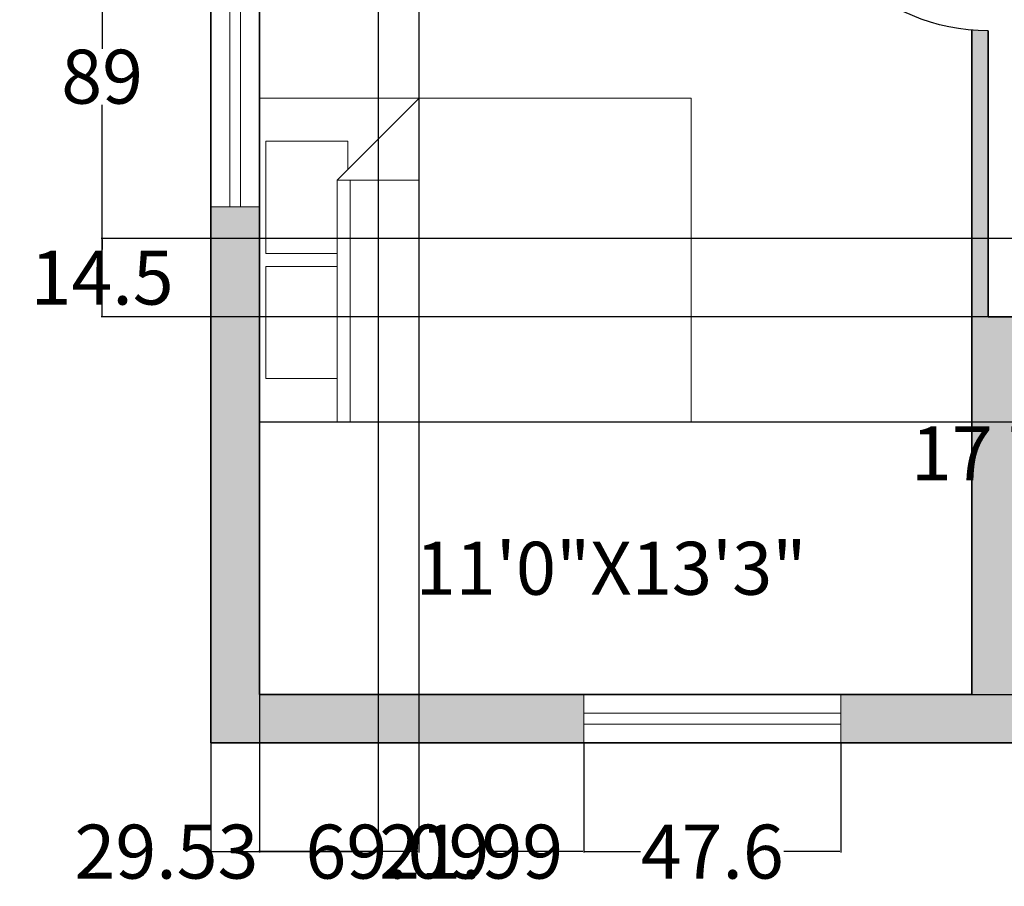
# Model space of a CAD drawing. Units: inches. Extents: x -75 to 484, y -248 to 214.
# Tile 1 of 7: x -20 to 162, y -248 to -87. Entities that reach past the tile are written whole.
import ezdxf

# ---------------------------------------------------------------- set-up
doc = ezdxf.new("R2010")
doc.units = ezdxf.units.IN
doc.header["$MEASUREMENT"] = 0
for name, color, linetype, lineweight in [('A-ANNO-DIMS', 2, 'Continuous', 18), ('A-AREA-IDEN', 7, 'Continuous', 18), ('A-DOOR', 3, 'Continuous', 25), ('A-FURN', 8, 'Continuous', 18), ('A-GLAZ', 4, 'Continuous', 18), ('A-WALL', 7, 'Continuous', 35)]:
    doc.layers.add(name, color=color, linetype=linetype, lineweight=lineweight)
doc.layers.add('A-WALL-PATT', color=252, linetype='Continuous', lineweight=9, true_color=0x939598)
doc.styles.get("Standard").update_dxf_attribs({"font": 'arial.ttf'})
doc.dimstyles.get("Standard").update_dxf_attribs({"dimtxt": 10, "dimasz": 0.18, "dimexe": 0.18, "dimexo": 0.0625, "dimgap": 0.09, "dimtad": 0, "dimtih": 1, "dimtoh": 1, "dimdec": 0, "dimzin": 0, "dimdsep": 46, "dimlunit": 3, "dimtxsty": 'Standard', "dimcen": 0.09, "dimadec": 0, "dimazin": 0, "dimtfac": 1, "dimtdec": 0, "dimtofl": 0, "dimtmove": 0, "dimatfit": 3, "dimfxl": 1, "dimtolj": 1, "dimtzin": 0, "dimarcsym": 0})

# ---------------------------------------------------------------- blocks, each defined once
blk = doc.blocks.new('Bed - Queen')
for p, q in [((0, -80.00003), (0, 0)), ((0, 0), (59.99999, 0)), ((59.99999, 0), (59.99999, -80.00003)), ((7.99999, -1.2), (28.79998, -1.2)), ((7.99999, -14.4), (7.99999, -1.2)), ((28.79998, -1.2), (28.79998, -14.4)), ((31.19999, -1.2), (51.99999, -1.2)), ((31.19999, -14.4), (31.19999, -1.2)), ((51.99999, -1.2), (51.99999, -16.4)), ((0, -14.4), (44.8, -14.4)), ((59.99999, -29.6), (44.8, -14.4)), ((44.8, -14.4), (44.8, -29.6)), ((51.99999, -16.4), (46.79936, -16.4)), ((44.8, -16.8), (0, -16.8)), ((44.8, -29.6), (59.99999, -29.6)), ((59.99999, -80.00003), (0, -80.00003))]:
    blk.add_line(p, q)
blk = doc.blocks.new('DOOR-SINGLE-36')
for p, q in [((35, 36), (35, 0)), ((36, 36), (36, 0))]:
    blk.add_line(p, q)
blk.add_arc((36, 36), 36, 180, 270)
blk = doc.blocks.new('WIN-48-NOM')
for p, q in [((9, 47.92), (0, 47.92)), ((3.5, 0), (3.5, 47.92)), ((5.5, 0), (5.5, 47.92)), ((0, 0), (9, 0))]:
    blk.add_line(p, q)
blk = doc.blocks.new('*D22')
at = {"layer": 'A-ANNO-DIMS', "color": 0, "lineweight": -2, "transparency": 16777216}
for p, q in [((190.41, -170.27), (192.32, -167.62)), ((192.07, -167.66), (191.89, -167.66)), ((192.22, -167.77), (192.07, -167.66)), ((206.13, -177.79), (192.36, -167.87)), ((204.48, -180.4), (206.39, -177.75))]:
    blk.add_line(p, q, dxfattribs=at)
at = {"layer": 'A-ANNO-DIMS', "color": 0, "transparency": 16777216}
for points in [[(192.38, -167.85), (192.34, -167.89), (192.22, -167.77)], [(206.15, -177.77), (206.12, -177.81), (206.28, -177.9)]]:
    blk.add_solid(points, dxfattribs=at)
at = {"layer": 'Defpoints', "color": 0, "transparency": 16777216}
for p in [(192.22, -167.77), (190.37, -170.32), (204.44, -180.45)]:
    blk.add_point(p, dxfattribs=at)
at = {"layer": 'A-ANNO-DIMS', "color": 0, "transparency": 16777216, "insert": (167.93, -167.66), "char_height": 10, "attachment_point": 5}
blk.add_mtext('\\A1;17 TYP.', dxfattribs=at)
blk = doc.blocks.new('*D27')
at = {"layer": 'A-ANNO-DIMS', "color": 0, "lineweight": -2, "transparency": 16777216}
for p, q in [((196.34, -31.46), (182.57, -31.46)), ((182.75, -31.64), (182.75, -71.7)), ((182.75, -122.28), (182.75, -82.22)), ((196.34, -122.46), (182.57, -122.46))]:
    blk.add_line(p, q, dxfattribs=at)
at = {"layer": 'A-ANNO-DIMS', "color": 0, "transparency": 16777216}
for points in [[(182.72, -31.64), (182.78, -31.64), (182.75, -31.46)], [(182.72, -122.28), (182.78, -122.28), (182.75, -122.46)]]:
    blk.add_solid(points, dxfattribs=at)
at = {"layer": 'Defpoints', "color": 0, "transparency": 16777216}
for p in [(196.4, -31.46), (182.75, -122.46), (196.4, -122.46)]:
    blk.add_point(p, dxfattribs=at)
at = {"layer": 'A-ANNO-DIMS', "color": 0, "transparency": 16777216, "insert": (182.75, -76.96), "char_height": 10, "attachment_point": 5}
blk.add_mtext('\\A1;DINING SET 91', dxfattribs=at)
blk = doc.blocks.new('*D48')
at = {"layer": 'A-ANNO-DIMS', "color": 0, "lineweight": -2, "transparency": 16777216}
for p, q in [((15.21, -221.41), (15.21, -241.67)), ((84.3, -221.41), (84.3, -241.67)), ((15.39, -241.49), (32.76, -241.49)), ((84.12, -241.49), (66.76, -241.49))]:
    blk.add_line(p, q, dxfattribs=at)
at = {"layer": 'A-ANNO-DIMS', "color": 0, "transparency": 16777216}
for points in [[(15.39, -241.46), (15.39, -241.52), (15.21, -241.49)], [(84.12, -241.46), (84.12, -241.52), (84.3, -241.49)]]:
    blk.add_solid(points, dxfattribs=at)
at = {"layer": 'Defpoints', "color": 0, "transparency": 16777216}
for p in [(15.21, -221.34), (84.3, -221.34), (84.3, -241.49)]:
    blk.add_point(p, dxfattribs=at)
at = {"layer": 'A-ANNO-DIMS', "color": 0, "transparency": 16777216, "insert": (49.76, -241.49), "char_height": 10, "attachment_point": 5}
blk.add_mtext('\\A1;69.09', dxfattribs=at)
blk = doc.blocks.new('*D49')
at = {"layer": 'A-ANNO-DIMS', "color": 0, "lineweight": -2, "transparency": 16777216}
for p, q in [((84.3, -221.41), (84.3, -241.67)), ((131.9, -221.41), (131.9, -241.67)), ((84.48, -241.49), (94.83, -241.49)), ((131.72, -241.49), (121.38, -241.49))]:
    blk.add_line(p, q, dxfattribs=at)
at = {"layer": 'A-ANNO-DIMS', "color": 0, "transparency": 16777216}
for points in [[(84.48, -241.46), (84.48, -241.52), (84.3, -241.49)], [(131.72, -241.46), (131.72, -241.52), (131.9, -241.49)]]:
    blk.add_solid(points, dxfattribs=at)
at = {"layer": 'Defpoints', "color": 0, "transparency": 16777216}
for p in [(84.3, -221.34), (131.9, -221.34), (131.9, -241.49)]:
    blk.add_point(p, dxfattribs=at)
at = {"layer": 'A-ANNO-DIMS', "color": 0, "transparency": 16777216, "insert": (108.1, -241.49), "char_height": 10, "attachment_point": 5}
blk.add_mtext('\\A1;47.6', dxfattribs=at)
blk = doc.blocks.new('*D58')
at = {"layer": 'A-ANNO-DIMS', "color": 0, "lineweight": -2, "transparency": 16777216}
for p, q in [((24.21, -53.41), (24.21, -241.67)), ((53.74, -53.41), (53.74, -241.67)), ((24.21, -241.49), (24.03, -241.49)), ((53.56, -241.49), (24.39, -241.49))]:
    blk.add_line(p, q, dxfattribs=at)
at = {"layer": 'A-ANNO-DIMS', "color": 0, "transparency": 16777216}
for points in [[(24.39, -241.46), (24.39, -241.52), (24.21, -241.49)], [(53.56, -241.46), (53.56, -241.52), (53.74, -241.49)]]:
    blk.add_solid(points, dxfattribs=at)
at = {"layer": 'Defpoints', "color": 0, "transparency": 16777216}
for p in [(24.21, -53.34), (53.74, -53.34), (24.21, -241.49)]:
    blk.add_point(p, dxfattribs=at)
at = {"layer": 'A-ANNO-DIMS', "color": 0, "transparency": 16777216, "insert": (6.98, -241.49), "char_height": 10, "attachment_point": 5}
blk.add_mtext('\\A1;29.53', dxfattribs=at)
blk = doc.blocks.new('*D68')
at = {"layer": 'A-ANNO-DIMS', "color": 0, "lineweight": -2, "transparency": 16777216}
for p, q in [((340.8, -127.84), (-5.12, -127.84)), ((-4.94, -128.02), (-4.94, -129.9)), ((-4.94, -142.16), (-4.94, -140.29)), ((340.8, -142.34), (-5.12, -142.34))]:
    blk.add_line(p, q, dxfattribs=at)
at = {"layer": 'A-ANNO-DIMS', "color": 0, "transparency": 16777216}
for points in [[(-4.97, -128.02), (-4.91, -128.02), (-4.94, -127.84)], [(-4.97, -142.16), (-4.91, -142.16), (-4.94, -142.34)]]:
    blk.add_solid(points, dxfattribs=at)
at = {"layer": 'Defpoints', "color": 0, "transparency": 16777216}
for p in [(340.87, -127.84), (-4.94, -142.34), (340.87, -142.34)]:
    blk.add_point(p, dxfattribs=at)
at = {"layer": 'A-ANNO-DIMS', "color": 0, "transparency": 16777216, "insert": (-4.94, -135.09), "char_height": 10, "attachment_point": 5}
blk.add_mtext('\\A1;14.5', dxfattribs=at)
blk = doc.blocks.new('*D69')
at = {"layer": 'A-ANNO-DIMS', "color": 0, "lineweight": -2, "transparency": 16777216}
for p, q in [((285.15, -53.34), (-5.12, -53.34)), ((-4.94, -53.52), (-4.94, -92.65)), ((-4.94, -142.16), (-4.94, -103.04)), ((285.15, -142.34), (-5.12, -142.34))]:
    blk.add_line(p, q, dxfattribs=at)
at = {"layer": 'A-ANNO-DIMS', "color": 0, "transparency": 16777216}
for points in [[(-4.97, -53.52), (-4.91, -53.52), (-4.94, -53.34)], [(-4.97, -142.16), (-4.91, -142.16), (-4.94, -142.34)]]:
    blk.add_solid(points, dxfattribs=at)
at = {"layer": 'Defpoints', "color": 0, "transparency": 16777216}
for p in [(285.21, -53.34), (-4.94, -142.34), (285.21, -142.34)]:
    blk.add_point(p, dxfattribs=at)
at = {"layer": 'A-ANNO-DIMS', "color": 0, "transparency": 16777216, "insert": (-4.94, -97.84), "char_height": 10, "attachment_point": 5}
blk.add_mtext('\\A1;89', dxfattribs=at)
blk = doc.blocks.new('*D74')
at = {"layer": 'A-ANNO-DIMS', "color": 0, "lineweight": -2, "transparency": 16777216}
for p, q in [((24.27, -161.82), (434.54, -161.82)), ((434.36, -162), (434.36, -181.88)), ((434.36, -212.16), (434.36, -192.28)), ((24.27, -212.34), (434.54, -212.34))]:
    blk.add_line(p, q, dxfattribs=at)
at = {"layer": 'A-ANNO-DIMS', "color": 0, "transparency": 16777216}
for points in [[(434.33, -162), (434.39, -162), (434.36, -161.82)], [(434.33, -212.16), (434.39, -212.16), (434.36, -212.34)]]:
    blk.add_solid(points, dxfattribs=at)
at = {"layer": 'Defpoints', "color": 0, "transparency": 16777216}
for p in [(24.21, -161.82), (434.36, -161.82), (24.21, -212.34)]:
    blk.add_point(p, dxfattribs=at)
at = {"layer": 'A-ANNO-DIMS', "color": 0, "transparency": 16777216, "insert": (434.36, -187.08), "char_height": 10, "attachment_point": 5}
blk.add_mtext('\\A1;50.53', dxfattribs=at)
blk = doc.blocks.new('*D76')
at = {"layer": 'A-ANNO-DIMS', "color": 0, "lineweight": -2, "transparency": 16777216}
for p, q in [((24.21, 138.59), (24.21, -241.67)), ((46.2, 104.59), (46.2, -241.67)), ((24.39, -241.49), (46.02, -241.49)), ((46.2, -241.49), (46.38, -241.49))]:
    blk.add_line(p, q, dxfattribs=at)
at = {"layer": 'A-ANNO-DIMS', "color": 0, "transparency": 16777216}
for points in [[(24.39, -241.46), (24.39, -241.52), (24.21, -241.49)], [(46.02, -241.46), (46.02, -241.52), (46.2, -241.49)]]:
    blk.add_solid(points, dxfattribs=at)
at = {"layer": 'Defpoints', "color": 0, "transparency": 16777216}
for p in [(24.21, 138.66), (46.2, 104.66), (46.2, -241.49)]:
    blk.add_point(p, dxfattribs=at)
at = {"layer": 'A-ANNO-DIMS', "color": 0, "transparency": 16777216, "insert": (63.44, -241.49), "char_height": 10, "attachment_point": 5}
blk.add_mtext('\\A1;21.99', dxfattribs=at)

msp = doc.modelspace()

# ---------------------------------------------------------------- hatches: boundary and pattern name
at = {"layer": 'A-WALL-PATT'}
h = msp.add_hatch(color=256, dxfattribs=at)
h.dxf.hatch_style = 1
h.paths.add_polyline_path([(184.9004, 147.6567), (15.2094, 147.6567), (15.2094, 92.5031), (24.2094, 92.5031), (24.2094, 138.6567), (186.0436, 138.6567, -0.06325422)])
h.paths.add_polyline_path([(414.2094, 147.6567), (249.2094, 147.6567), (220.9004, 147.6567), (220.9004, 138.6567), (240.2094, 138.6567), (240.2094, 18.6567), (240.2094, 9.6567), (249.2094, 9.6567), (249.2094, 45.6567), (249.2094, 138.6567), (405.2094, 138.6567), (405.2094, 98.3029), (414.2094, 98.3029)])
h.paths.add_polyline_path([(159.2094, 18.6567), (24.2094, 18.6567), (24.2094, 44.5861), (15.2094, 44.5861), (15.2094, 9.6567), (15.2094, -3.1791), (24.2094, -3.1791), (24.2094, 9.6567), (132.2094, 9.6567), (132.2094, -50.3433), (83.7394, -50.3433), (83.7394, -53.3433), (132.2094, -53.3433), (159.2094, -53.3433), (159.2094, -50.3433), (135.2094, -50.3433), (135.2094, 9.6567), (159.2094, 9.6567)])
h.paths.add_polyline_path([(53.8898, -50.3433), (24.2094, -50.3433), (24.2094, -27.303), (15.2094, -27.303), (15.2094, -50.3433), (15.2094, -53.3433), (15.2094, -74.0487), (24.2094, -74.0487), (24.2094, -53.3433), (53.7394, -53.3433, -0.02504709)])
h.paths.add_polyline_path([(24.2094, -121.9657), (15.2094, -121.9657), (15.2094, -212.3433), (15.2094, -221.3433), (24.2094, -221.3433), (84.3017, -221.3433), (84.3017, -212.3433), (24.2094, -212.3433)])
h.paths.add_polyline_path([(414.2094, -155.3433), (414.2094, -53.3433), (414.2094, -50.3433), (414.2094, -36.8417), (405.2094, -36.8417), (405.2094, -50.3433), (309.2094, -50.3433), (309.2094, 16.0463), (324.2573, 16.0463), (324.2573, 18.6567), (284.0663, 18.6567, -0.06325422), (285.2094, 9.6567), (306.2094, 9.6567), (306.2094, -50.3433), (285.2094, -50.3433), (285.2094, -53.3433), (309.2094, -53.3433), (405.2094, -53.3433), (405.2094, -212.3433), (293.2094, -212.3433), (293.2094, -158.3433), (293.2094, -145.3433), (300.0339, -145.3433), (300.0339, -142.3433), (285.2094, -142.3433), (159.2094, -142.3433), (159.2094, -89.3433, -0.02086055), (156.2094, -89.218), (156.2094, -212.3433), (131.9001, -212.3433), (131.9001, -221.3433), (156.2094, -221.3433), (165.2094, -221.3433), (285.2094, -221.3433), (288.6713, -221.3433), (293.2094, -221.3433), (405.2094, -221.3433), (414.2094, -221.3433)])
h.paths.add_polyline_path([(165.2094, -212.3433), (165.2094, -151.3433), (285.2094, -151.3433), (285.2094, -212.3433)], flags=16)
h.paths.add_polyline_path([(189.462, -195.5437), (182.159, -190.2838, -0.23606798), (182.5164, -188.0765), (181.7049, -187.4921), (185.5037, -182.2177), (184.648, -181.6013, -0.04492589), (180.0821, -186.3232), (179.2706, -185.7388), (189.206, -171.9443), (190.0174, -172.5287, -0.04492589), (186.9857, -178.3556), (187.8415, -178.9719), (191.6403, -173.6976), (192.4517, -174.282, -0.23606798), (194.432, -173.2435), (201.735, -178.5034, -0.23606798), (201.3776, -180.7107), (202.189, -181.2952, -0.11764706), (192.2537, -195.0897), (191.4423, -194.5053, -0.23606798)], flags=0)
h.paths.add_polyline_path([(253.751, -177.9543), (254.5293, -177.3263, -0.23606798), (254.0517, -175.1419), (261.056, -169.4904, -0.23606798), (263.0902, -170.419), (263.8684, -169.7911), (267.95, -174.8498), (268.7708, -174.1875, -0.04492589), (265.425, -168.5352), (266.2032, -167.9073), (276.8782, -181.1378), (276.0999, -181.7657, -0.04492589), (271.2826, -177.3006), (270.4618, -177.9629), (274.5434, -183.0216), (273.7651, -183.6495, -0.23606798), (274.2427, -185.834), (267.2383, -191.4854, -0.23606798), (265.2042, -190.5568), (264.4259, -191.1848, -0.11764706)], flags=0)
h.paths.add_polyline_path([(405.2094, -142.3433), (336.0339, -142.3433, -0.02086055), (335.9087, -145.3433), (405.2094, -145.3433)], flags=17)
h.paths.add_polyline_path([(414.2094, 50.4831), (405.2094, 50.4831), (405.2094, 18.6567), (354.2573, 18.6567, -0.02178446), (354.1435, 16.0463), (405.2094, 16.0463), (405.2094, -14.6494), (414.2094, -14.6494), (414.2094, 9.6567)])
h.paths.add_polyline_path([(200.2091, -179.9247), (255.2702, -179.9247), (255.2702, -168.0448), (200.2091, -168.0448)], flags=8)
h.paths.add_polyline_path([(200.2352, -167.6036), (249.7883, -167.6036), (249.7883, -155.8804), (200.2352, -155.8804)], flags=8)

# ---------------------------------------------------------------- linework, layer by layer
at = {"layer": 'A-GLAZ'}
for p, q in [((84.3017, -216.8433), (84.3017, -212.3433)), ((84.3017, -212.3433), (84.3017, -221.3433)), ((131.9001, -212.3433), (131.9001, -221.3433)), ((131.9001, -215.8433), (84.3017, -215.8433)), ((131.9001, -217.8433), (84.3017, -217.8433))]:
    msp.add_line(p, q, dxfattribs=at)
at = {"layer": 'A-WALL'}
for p, q in [((15.2094, -53.3433), (15.2094, -212.3433)), ((24.2094, -53.3433), (24.2094, -212.3433)), ((156.2094, -212.3433), (156.2094, -89.218)), ((159.2094, -89.3433), (159.2094, -142.3433)), ((159.2094, -142.3433), (285.2094, -142.3433)), ((15.2094, -212.3433), (15.2094, -221.3433)), ((24.2094, -212.3433), (156.2094, -212.3433)), ((15.2094, -221.3433), (24.2094, -221.3433)), ((24.2094, -221.3433), (156.2094, -221.3433)), ((165.2094, -221.3433), (156.2094, -221.3433))]:
    msp.add_line(p, q, dxfattribs=at)

# ---------------------------------------------------------------- block references
at = {"layer": 'A-DOOR', "extrusion": (0, 0, -1), "zscale": -1, "rotation": 90.00000000000014}
msp.add_blockref('DOOR-SINGLE-36', (-123.2094, -89.3433), dxfattribs=at)
at = {"layer": 'A-FURN', "rotation": 90}
msp.add_blockref('Bed - Queen', (24.2094, -161.8152), dxfattribs=at)
at = {"layer": 'A-GLAZ', "rotation": 180}
msp.add_blockref('WIN-48-NOM', (24.2094, -74.0487), dxfattribs=at)

# ---------------------------------------------------------------- texts
at = {"layer": 'A-AREA-IDEN'}
msp.add_text('11\'0"X13\'3"', height=9.820584, dxfattribs=at).set_placement((53.1237, -193.8743))

# ---------------------------------------------------------------- dimensions: what is measured, and where the dimension line sits
at = {"layer": 'A-ANNO-DIMS'}
for base, p1, p2, override, picture, middle in [((46.1998, -241.4933), (24.2094, 138.6567), (46.1998, 104.6567), {"dimdec": 2, "dimlfac": 1, "dimrnd": 0, "dimzin": 0, "dimdsep": 46, "dimlunit": 2}, '*D76', (63.4378, -241.4933)), ((24.2094, -241.4933), (53.7394, -53.3433), (24.2094, -53.3433), {"dimdec": 2, "dimlfac": 1, "dimrnd": 0, "dimzin": 0, "dimdsep": 46, "dimlunit": 2}, '*D58', (6.9817, -241.4933)), ((84.3017, -241.4933), (15.2094, -221.3433), (84.3017, -221.3433), {"dimdec": 2, "dimlfac": 1, "dimrnd": 0, "dimzin": 0, "dimdsep": 46, "dimlunit": 2}, '*D48', (49.7555, -241.4933)), ((131.9001, -241.4933), (84.3017, -221.3433), (131.9001, -221.3433), {"dimdec": 1, "dimlfac": 1, "dimrnd": 0, "dimzin": 0, "dimdsep": 46, "dimlunit": 2}, '*D49', (108.1009, -241.4933))]:
    dim = msp.add_linear_dim(base=base, p1=p1, p2=p2, dimstyle='Standard', override=override, dxfattribs=at)
    dim.commit()
    dim.dimension.update_dxf_attribs({"geometry": picture, "text_midpoint": middle})
for base, p1, p2, angle, text, picture, middle in [((182.7486, -122.4627), (196.3986, -31.4627), (196.3986, -122.4627), 270, 'DINING SET <>', '*D27', (182.7486, -76.9627)), ((192.2158, -167.7653), (204.4398, -180.4515), (190.3748, -170.3214), 144.237146, '<> TYP.', '*D22', (167.932, -167.6601))]:
    dim = msp.add_linear_dim(base=base, p1=p1, p2=p2, angle=angle, text=text, dimstyle='Standard', override={"dimdec": 0, "dimlfac": 1, "dimrnd": 0, "dimzin": 0, "dimdsep": 46, "dimlunit": 2}, dxfattribs=at)
    dim.commit()
    dim.dimension.update_dxf_attribs({"geometry": picture, "text_midpoint": middle})
for base, p1, p2, override, picture, middle in [((-4.9406, -142.3433), (285.2094, -53.3433), (285.2094, -142.3433), {"dimdec": 0, "dimlfac": 1, "dimrnd": 0, "dimzin": 0, "dimdsep": 46, "dimlunit": 2}, '*D69', (-4.9406, -97.8433)), ((-4.9406, -142.3433), (340.8661, -127.8437), (340.8661, -142.3433), {"dimdec": 1, "dimlfac": 1, "dimrnd": 0, "dimzin": 0, "dimdsep": 46, "dimlunit": 2}, '*D68', (-4.9406, -135.0935)), ((434.3594, -161.8152), (24.2094, -212.3433), (24.2094, -161.8152), {"dimdec": 2, "dimlfac": 1, "dimrnd": 0, "dimzin": 0, "dimdsep": 46, "dimlunit": 2}, '*D74', (434.3594, -187.0792))]:
    dim = msp.add_linear_dim(base=base, p1=p1, p2=p2, angle=90, dimstyle='Standard', override=override, dxfattribs=at)
    dim.commit()
    dim.dimension.update_dxf_attribs({"geometry": picture, "text_midpoint": middle})

doc.saveas('drawing.dxf')
